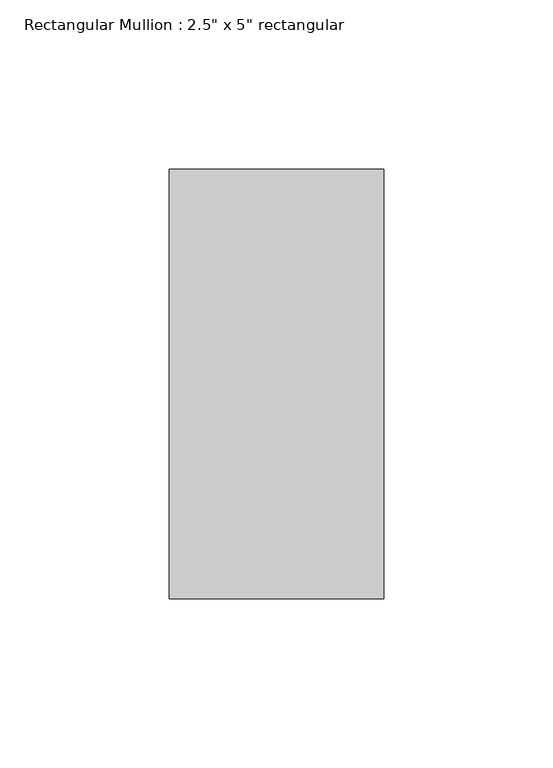
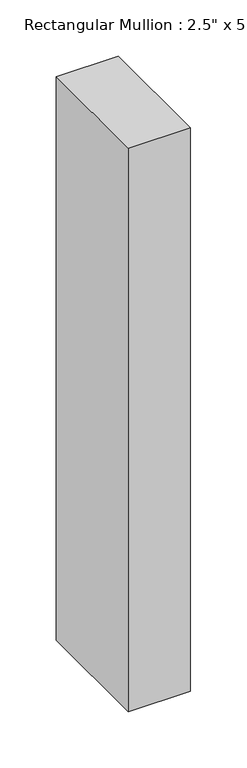
"""IFC4 building model written with IfcOpenShell, lengths in millimetres: member geometry."""

from ifc_helpers import new_model, si_unit, frame, origin, place, context, project, spatial, polyline, outline, extrude, source, transform, mapped, element, save


def member_47bfaf8a(model_context):
    return source(origin(), model_context, "Body", "SweptSolid", [
        extrude(outline(polyline([(0.0, 63.5), (0.0, -63.5), (-63.5, -63.5), (-63.5, 63.5), (0.0, 63.5)])), frame((0.0, 0.0, -609.6), z_axis=(0.0, 0.0, 1.0), x_axis=(1.0, 0.0, 0.0)), (0.0, 0.0, 1.0), 609.6),
    ])


if __name__ == "__main__":
    model = new_model("IFC4")
    model_context = context("Model", 3, world=origin())
    ifc_project = project(units=[si_unit("LENGTHUNIT", "METRE", prefix="MILLI")], contexts=[model_context])
    site = spatial("IfcSite", under=ifc_project)
    building = spatial("IfcBuilding", under=site)
    placement = place(None, origin())
    member_shape = member_47bfaf8a(model_context)
    element("IfcMember", 1, ObjectType="Rectangular Mullion : 2.5\" x 5\" rectangular", at=placement, inside=building, context=model_context, shape_type="MappedRepresentation", body=[
        mapped(member_shape, transform((0.0, 0.0, 0.0), x_axis=(1.0, 0.0, 0.0), y_axis=(0.0, 1.0, 0.0), z_axis=(0.0, 0.0, 1.0))),
    ])
    save(model, "model.ifc")

# Revit data of these elements
# Type "Rectangular Mullion : 2.5\" x 5\" rectangular"
#   built-in parameter 1007304 = 0.416667 (stored number, unit not read)
#   built-in parameter 1007301 = 0.104167 (stored number, unit not read)
#   built-in parameter 1007300 = 0.104167 (stored number, unit not read)
